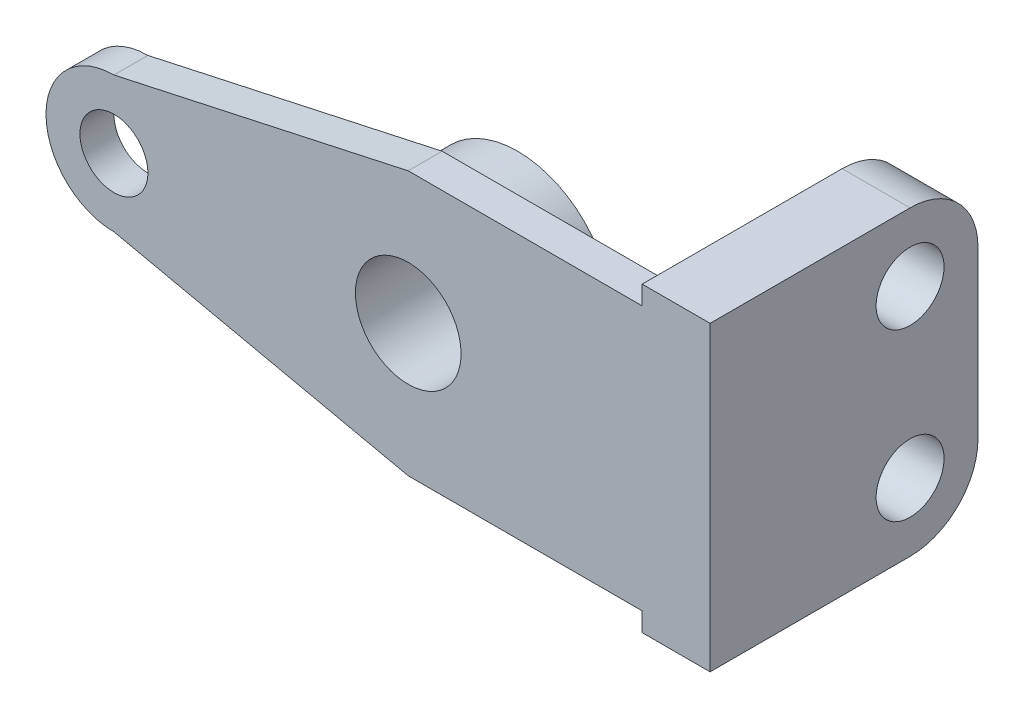
ISO-10303-21;
HEADER;
FILE_DESCRIPTION(('STEP AP214'),'2;1');
FILE_NAME('part.step','',(''),(''),'','','');
FILE_SCHEMA(('AUTOMOTIVE_DESIGN { 1 0 10303 214 1 1 1 1 }'));
ENDSEC;
DATA;
#1=APPLICATION_CONTEXT('core data for automotive mechanical design processes');
#2=APPLICATION_PROTOCOL_DEFINITION('international standard','automotive_design',2000,#1);
#3=PRODUCT_CONTEXT('',#1,'mechanical');
#4=PRODUCT('Part','Part','',(#3));
#5=PRODUCT_RELATED_PRODUCT_CATEGORY('part','',(#4));
#6=PRODUCT_DEFINITION_FORMATION('','',#4);
#7=PRODUCT_DEFINITION_CONTEXT('part definition',#1,'design');
#8=PRODUCT_DEFINITION('design','',#6,#7);
#9=PRODUCT_DEFINITION_SHAPE('','',#8);
#10=(LENGTH_UNIT() NAMED_UNIT(*) SI_UNIT(.MILLI.,.METRE.));
#11=(NAMED_UNIT(*) PLANE_ANGLE_UNIT() SI_UNIT($,.RADIAN.));
#12=(NAMED_UNIT(*) SI_UNIT($,.STERADIAN.) SOLID_ANGLE_UNIT());
#13=UNCERTAINTY_MEASURE_WITH_UNIT(LENGTH_MEASURE(1.E-05),#10,'distance_accuracy_value','');
#14=(GEOMETRIC_REPRESENTATION_CONTEXT(3) GLOBAL_UNCERTAINTY_ASSIGNED_CONTEXT((#13)) GLOBAL_UNIT_ASSIGNED_CONTEXT((#10,
#11,#12)) REPRESENTATION_CONTEXT('',''));
#15=CARTESIAN_POINT('',(0.,0.,0.));
#16=DIRECTION('',(0.,0.,1.));
#17=DIRECTION('',(1.,0.,0.));
#18=AXIS2_PLACEMENT_3D('',#15,#16,#17);
#19=CARTESIAN_POINT('',(-14.5645692766358,66.8256707986819,9.));
#20=DIRECTION('',(-0.212949665458365,0.977063170926614,0.));
#21=DIRECTION('',(-0.977063170926615,-0.212949665458365,0.));
#22=AXIS2_PLACEMENT_3D('',#19,#20,#21);
#23=PLANE('',#22);
#24=DIRECTION('',(0.977063170926614,0.212949665458365,0.));
#25=VECTOR('',#24,1.);
#26=CARTESIAN_POINT('',(-14.5645692766358,66.8256707986819,0.));
#27=LINE('',#26,#25);
#28=CARTESIAN_POINT('',(-78.,53.,0.));
#29=VERTEX_POINT('',#28);
#30=CARTESIAN_POINT('',(0.,70.,0.));
#31=VERTEX_POINT('',#30);
#32=EDGE_CURVE('E206',#29,#31,#27,.T.);
#33=ORIENTED_EDGE('',*,*,#32,.F.);
#34=DIRECTION('',(0.,0.,-1.));
#35=VECTOR('',#34,1.);
#36=CARTESIAN_POINT('',(-78.,53.,9.));
#37=LINE('',#36,#35);
#38=CARTESIAN_POINT('',(-78.,53.,9.));
#39=VERTEX_POINT('',#38);
#40=EDGE_CURVE('E245',#39,#29,#37,.T.);
#41=ORIENTED_EDGE('',*,*,#40,.F.);
#42=DIRECTION('',(0.977063170926614,0.212949665458365,0.));
#43=VECTOR('',#42,1.);
#44=CARTESIAN_POINT('',(-14.5645692766358,66.8256707986819,9.));
#45=LINE('',#44,#43);
#46=CARTESIAN_POINT('',(0.,70.,9.));
#47=VERTEX_POINT('',#46);
#48=EDGE_CURVE('E207',#39,#47,#45,.T.);
#49=ORIENTED_EDGE('',*,*,#48,.T.);
#50=DIRECTION('',(0.,0.,-1.));
#51=VECTOR('',#50,1.);
#52=CARTESIAN_POINT('',(0.,70.,9.));
#53=LINE('',#52,#51);
#54=EDGE_CURVE('E222',#47,#31,#53,.T.);
#55=ORIENTED_EDGE('',*,*,#54,.T.);
#56=EDGE_LOOP('',(#33,#41,#49,#55));
#57=FACE_BOUND('',#56,.T.);
#58=ADVANCED_FACE('F41',(#57),#23,.T.);
#59=CARTESIAN_POINT('',(-78.,35.,9.));
#60=DIRECTION('',(0.,0.,-1.));
#61=DIRECTION('',(-1.,0.,0.));
#62=AXIS2_PLACEMENT_3D('',#59,#60,#61);
#63=CYLINDRICAL_SURFACE('',#62,18.);
#64=CARTESIAN_POINT('',(-78.,35.,0.));
#65=DIRECTION('',(0.,0.,1.));
#66=DIRECTION('',(1.,0.,0.));
#67=AXIS2_PLACEMENT_3D('',#64,#65,#66);
#68=CIRCLE('',#67,18.);
#69=CARTESIAN_POINT('',(-78.,17.,0.));
#70=VERTEX_POINT('',#69);
#71=EDGE_CURVE('E221',#29,#70,#68,.T.);
#72=ORIENTED_EDGE('',*,*,#71,.T.);
#73=DIRECTION('',(0.,0.,-1.));
#74=VECTOR('',#73,1.);
#75=CARTESIAN_POINT('',(-78.,17.,9.));
#76=LINE('',#75,#74);
#77=CARTESIAN_POINT('',(-78.,17.,9.));
#78=VERTEX_POINT('',#77);
#79=EDGE_CURVE('E239',#78,#70,#76,.T.);
#80=ORIENTED_EDGE('',*,*,#79,.F.);
#81=CARTESIAN_POINT('',(-78.,35.,9.));
#82=DIRECTION('',(0.,0.,1.));
#83=DIRECTION('',(1.,0.,0.));
#84=AXIS2_PLACEMENT_3D('',#81,#82,#83);
#85=CIRCLE('',#84,18.);
#86=EDGE_CURVE('E215',#39,#78,#85,.T.);
#87=ORIENTED_EDGE('',*,*,#86,.F.);
#88=ORIENTED_EDGE('',*,*,#40,.T.);
#89=EDGE_LOOP('',(#72,#80,#87,#88));
#90=FACE_BOUND('',#89,.T.);
#91=ADVANCED_FACE('F289',(#90),#63,.T.);
#92=CARTESIAN_POINT('',(0.,0.,9.));
#93=DIRECTION('',(0.212949665458365,0.977063170926614,0.));
#94=DIRECTION('',(-0.977063170926615,0.212949665458365,0.));
#95=AXIS2_PLACEMENT_3D('',#92,#93,#94);
#96=PLANE('',#95);
#97=DIRECTION('',(0.977063170926614,-0.212949665458365,0.));
#98=VECTOR('',#97,1.);
#99=CARTESIAN_POINT('',(0.,0.,0.));
#100=LINE('',#99,#98);
#101=CARTESIAN_POINT('',(0.,0.,0.));
#102=VERTEX_POINT('',#101);
#103=EDGE_CURVE('E227',#70,#102,#100,.T.);
#104=ORIENTED_EDGE('',*,*,#103,.T.);
#105=DIRECTION('',(0.,0.,-1.));
#106=VECTOR('',#105,1.);
#107=CARTESIAN_POINT('',(0.,0.,9.));
#108=LINE('',#107,#106);
#109=CARTESIAN_POINT('',(0.,0.,9.));
#110=VERTEX_POINT('',#109);
#111=EDGE_CURVE('E237',#110,#102,#108,.T.);
#112=ORIENTED_EDGE('',*,*,#111,.F.);
#113=DIRECTION('',(0.977063170926614,-0.212949665458365,0.));
#114=VECTOR('',#113,1.);
#115=CARTESIAN_POINT('',(0.,0.,9.));
#116=LINE('',#115,#114);
#117=EDGE_CURVE('E214',#78,#110,#116,.T.);
#118=ORIENTED_EDGE('',*,*,#117,.F.);
#119=ORIENTED_EDGE('',*,*,#79,.T.);
#120=EDGE_LOOP('',(#104,#112,#118,#119));
#121=FACE_BOUND('',#120,.T.);
#122=ADVANCED_FACE('F292',(#121),#96,.F.);
#123=CARTESIAN_POINT('',(0.,0.,9.));
#124=DIRECTION('',(0.,1.,0.));
#125=DIRECTION('',(0.,0.,1.));
#126=AXIS2_PLACEMENT_3D('',#123,#124,#125);
#127=PLANE('',#126);
#128=DIRECTION('',(1.,0.,0.));
#129=VECTOR('',#128,1.);
#130=CARTESIAN_POINT('',(0.,0.,0.));
#131=LINE('',#130,#129);
#132=CARTESIAN_POINT('',(62.,0.,0.));
#133=VERTEX_POINT('',#132);
#134=EDGE_CURVE('E228',#102,#133,#131,.T.);
#135=ORIENTED_EDGE('',*,*,#134,.T.);
#136=DIRECTION('',(0.,0.,1.));
#137=VECTOR('',#136,1.);
#138=CARTESIAN_POINT('',(62.,0.,9.));
#139=LINE('',#138,#137);
#140=CARTESIAN_POINT('',(62.,0.,9.));
#141=VERTEX_POINT('',#140);
#142=EDGE_CURVE('E63',#133,#141,#139,.T.);
#143=ORIENTED_EDGE('',*,*,#142,.T.);
#144=DIRECTION('',(1.,0.,0.));
#145=VECTOR('',#144,1.);
#146=CARTESIAN_POINT('',(0.,0.,9.));
#147=LINE('',#146,#145);
#148=EDGE_CURVE('E136',#110,#141,#147,.T.);
#149=ORIENTED_EDGE('',*,*,#148,.F.);
#150=ORIENTED_EDGE('',*,*,#111,.T.);
#151=EDGE_LOOP('',(#135,#143,#149,#150));
#152=FACE_BOUND('',#151,.T.);
#153=ADVANCED_FACE('F305',(#152),#127,.F.);
#154=CARTESIAN_POINT('',(80.,0.,9.));
#155=DIRECTION('',(1.,0.,0.));
#156=DIRECTION('',(0.,0.,-1.));
#157=AXIS2_PLACEMENT_3D('',#154,#155,#156);
#158=PLANE('',#157);
#159=CARTESIAN_POINT('',(80.,57.,-44.));
#160=DIRECTION('',(1.,0.,0.));
#161=DIRECTION('',(0.,0.,-1.));
#162=AXIS2_PLACEMENT_3D('',#159,#160,#161);
#163=CIRCLE('',#162,9.);
#164=CARTESIAN_POINT('',(80.,57.,-53.));
#165=VERTEX_POINT('',#164);
#166=EDGE_CURVE('E452',#165,#165,#163,.T.);
#167=ORIENTED_EDGE('',*,*,#166,.F.);
#168=EDGE_LOOP('',(#167));
#169=FACE_BOUND('',#168,.T.);
#170=CARTESIAN_POINT('',(80.,13.,-44.));
#171=DIRECTION('',(1.,0.,0.));
#172=DIRECTION('',(0.,0.,-1.));
#173=AXIS2_PLACEMENT_3D('',#170,#171,#172);
#174=CIRCLE('',#173,9.);
#175=CARTESIAN_POINT('',(80.,13.,-53.));
#176=VERTEX_POINT('',#175);
#177=EDGE_CURVE('E457',#176,#176,#174,.T.);
#178=ORIENTED_EDGE('',*,*,#177,.F.);
#179=EDGE_LOOP('',(#178));
#180=FACE_BOUND('',#179,.T.);
#181=DIRECTION('',(0.,0.,-1.));
#182=VECTOR('',#181,1.);
#183=CARTESIAN_POINT('',(80.,-5.,9.));
#184=LINE('',#183,#182);
#185=CARTESIAN_POINT('',(80.,-5.,9.));
#186=VERTEX_POINT('',#185);
#187=CARTESIAN_POINT('',(80.,-5.,-44.));
#188=VERTEX_POINT('',#187);
#189=EDGE_CURVE('E146',#186,#188,#184,.T.);
#190=ORIENTED_EDGE('',*,*,#189,.T.);
#191=CARTESIAN_POINT('',(80.,13.,-44.));
#192=DIRECTION('',(1.,0.,0.));
#193=DIRECTION('',(0.,0.,1.));
#194=AXIS2_PLACEMENT_3D('',#191,#192,#193);
#195=CIRCLE('',#194,18.);
#196=CARTESIAN_POINT('',(80.,13.,-62.));
#197=VERTEX_POINT('',#196);
#198=EDGE_CURVE('E168',#188,#197,#195,.T.);
#199=ORIENTED_EDGE('',*,*,#198,.T.);
#200=DIRECTION('',(0.,1.,0.));
#201=VECTOR('',#200,1.);
#202=CARTESIAN_POINT('',(80.,57.,-62.));
#203=LINE('',#202,#201);
#204=CARTESIAN_POINT('',(80.,57.,-62.));
#205=VERTEX_POINT('',#204);
#206=EDGE_CURVE('E173',#197,#205,#203,.T.);
#207=ORIENTED_EDGE('',*,*,#206,.T.);
#208=CARTESIAN_POINT('',(80.,57.,-44.));
#209=DIRECTION('',(1.,0.,0.));
#210=DIRECTION('',(0.,0.,1.));
#211=AXIS2_PLACEMENT_3D('',#208,#209,#210);
#212=CIRCLE('',#211,18.);
#213=CARTESIAN_POINT('',(80.,75.,-44.));
#214=VERTEX_POINT('',#213);
#215=EDGE_CURVE('E143',#205,#214,#212,.T.);
#216=ORIENTED_EDGE('',*,*,#215,.T.);
#217=DIRECTION('',(0.,0.,-1.));
#218=VECTOR('',#217,1.);
#219=CARTESIAN_POINT('',(80.,75.,9.));
#220=LINE('',#219,#218);
#221=CARTESIAN_POINT('',(80.,75.,9.));
#222=VERTEX_POINT('',#221);
#223=EDGE_CURVE('E235',#222,#214,#220,.T.);
#224=ORIENTED_EDGE('',*,*,#223,.F.);
#225=DIRECTION('',(0.,-1.,0.));
#226=VECTOR('',#225,1.);
#227=CARTESIAN_POINT('',(80.,0.,9.));
#228=LINE('',#227,#226);
#229=EDGE_CURVE('E217',#222,#186,#228,.T.);
#230=ORIENTED_EDGE('',*,*,#229,.T.);
#231=EDGE_LOOP('',(#190,#199,#207,#216,#224,#230));
#232=FACE_BOUND('',#231,.T.);
#233=ADVANCED_FACE('F274',(#169,#180,#232),#158,.T.);
#234=CARTESIAN_POINT('',(0.,70.,9.));
#235=DIRECTION('',(0.,1.,0.));
#236=DIRECTION('',(0.,0.,1.));
#237=AXIS2_PLACEMENT_3D('',#234,#235,#236);
#238=PLANE('',#237);
#239=DIRECTION('',(0.,0.,1.));
#240=VECTOR('',#239,1.);
#241=CARTESIAN_POINT('',(62.,70.,9.));
#242=LINE('',#241,#240);
#243=CARTESIAN_POINT('',(62.,70.,0.));
#244=VERTEX_POINT('',#243);
#245=CARTESIAN_POINT('',(62.,70.,9.));
#246=VERTEX_POINT('',#245);
#247=EDGE_CURVE('E185',#244,#246,#242,.T.);
#248=ORIENTED_EDGE('',*,*,#247,.F.);
#249=DIRECTION('',(1.,0.,0.));
#250=VECTOR('',#249,1.);
#251=CARTESIAN_POINT('',(0.,70.,0.));
#252=LINE('',#251,#250);
#253=EDGE_CURVE('E213',#31,#244,#252,.T.);
#254=ORIENTED_EDGE('',*,*,#253,.F.);
#255=ORIENTED_EDGE('',*,*,#54,.F.);
#256=DIRECTION('',(1.,0.,0.));
#257=VECTOR('',#256,1.);
#258=CARTESIAN_POINT('',(0.,70.,9.));
#259=LINE('',#258,#257);
#260=EDGE_CURVE('E54',#47,#246,#259,.T.);
#261=ORIENTED_EDGE('',*,*,#260,.T.);
#262=EDGE_LOOP('',(#248,#254,#255,#261));
#263=FACE_BOUND('',#262,.T.);
#264=ADVANCED_FACE('F294',(#263),#238,.T.);
#265=CARTESIAN_POINT('',(0.,0.,9.));
#266=DIRECTION('',(0.,0.,1.));
#267=DIRECTION('',(1.,0.,0.));
#268=AXIS2_PLACEMENT_3D('',#265,#266,#267);
#269=PLANE('',#268);
#270=ORIENTED_EDGE('',*,*,#229,.F.);
#271=DIRECTION('',(1.,0.,0.));
#272=VECTOR('',#271,1.);
#273=CARTESIAN_POINT('',(62.,75.,9.));
#274=LINE('',#273,#272);
#275=CARTESIAN_POINT('',(62.,75.,9.));
#276=VERTEX_POINT('',#275);
#277=EDGE_CURVE('E178',#276,#222,#274,.T.);
#278=ORIENTED_EDGE('',*,*,#277,.F.);
#279=DIRECTION('',(0.,-1.,0.));
#280=VECTOR('',#279,1.);
#281=CARTESIAN_POINT('',(62.,-5.,9.));
#282=LINE('',#281,#280);
#283=EDGE_CURVE('E137',#276,#246,#282,.T.);
#284=ORIENTED_EDGE('',*,*,#283,.T.);
#285=ORIENTED_EDGE('',*,*,#260,.F.);
#286=ORIENTED_EDGE('',*,*,#48,.F.);
#287=ORIENTED_EDGE('',*,*,#86,.T.);
#288=ORIENTED_EDGE('',*,*,#117,.T.);
#289=ORIENTED_EDGE('',*,*,#148,.T.);
#290=CARTESIAN_POINT('',(62.,-5.,9.));
#291=VERTEX_POINT('',#290);
#292=EDGE_CURVE('E128',#141,#291,#282,.T.);
#293=ORIENTED_EDGE('',*,*,#292,.T.);
#294=DIRECTION('',(1.,0.,0.));
#295=VECTOR('',#294,1.);
#296=CARTESIAN_POINT('',(62.,-5.,9.));
#297=LINE('',#296,#295);
#298=EDGE_CURVE('E131',#291,#186,#297,.T.);
#299=ORIENTED_EDGE('',*,*,#298,.T.);
#300=EDGE_LOOP('',(#270,#278,#284,#285,#286,#287,#288,#289,#293,#299));
#301=FACE_BOUND('',#300,.T.);
#302=CARTESIAN_POINT('',(0.,35.,9.));
#303=DIRECTION('',(0.,0.,-1.));
#304=DIRECTION('',(-1.,0.,0.));
#305=AXIS2_PLACEMENT_3D('',#302,#303,#304);
#306=CIRCLE('',#305,14.);
#307=CARTESIAN_POINT('',(-14.,35.,9.));
#308=VERTEX_POINT('',#307);
#309=EDGE_CURVE('E193',#308,#308,#306,.T.);
#310=ORIENTED_EDGE('',*,*,#309,.T.);
#311=EDGE_LOOP('',(#310));
#312=FACE_BOUND('',#311,.T.);
#313=CARTESIAN_POINT('',(-78.,35.,9.));
#314=DIRECTION('',(0.,0.,-1.));
#315=DIRECTION('',(-1.,0.,0.));
#316=AXIS2_PLACEMENT_3D('',#313,#314,#315);
#317=CIRCLE('',#316,9.);
#318=CARTESIAN_POINT('',(-87.,35.,9.));
#319=VERTEX_POINT('',#318);
#320=EDGE_CURVE('E201',#319,#319,#317,.T.);
#321=ORIENTED_EDGE('',*,*,#320,.T.);
#322=EDGE_LOOP('',(#321));
#323=FACE_BOUND('',#322,.T.);
#324=ADVANCED_FACE('F133',(#301,#312,#323),#269,.T.);
#325=CARTESIAN_POINT('',(0.,0.,0.));
#326=DIRECTION('',(0.,0.,1.));
#327=DIRECTION('',(1.,0.,0.));
#328=AXIS2_PLACEMENT_3D('',#325,#326,#327);
#329=PLANE('',#328);
#330=CARTESIAN_POINT('',(0.,35.,0.));
#331=DIRECTION('',(0.,0.,1.));
#332=DIRECTION('',(1.,0.,0.));
#333=AXIS2_PLACEMENT_3D('',#330,#331,#332);
#334=CIRCLE('',#333,25.);
#335=CARTESIAN_POINT('',(25.,35.,0.));
#336=VERTEX_POINT('',#335);
#337=EDGE_CURVE('E48',#336,#336,#334,.F.);
#338=ORIENTED_EDGE('',*,*,#337,.F.);
#339=EDGE_LOOP('',(#338));
#340=FACE_BOUND('',#339,.T.);
#341=CARTESIAN_POINT('',(-78.,35.,0.));
#342=DIRECTION('',(0.,0.,-1.));
#343=DIRECTION('',(-1.,0.,0.));
#344=AXIS2_PLACEMENT_3D('',#341,#342,#343);
#345=CIRCLE('',#344,9.);
#346=CARTESIAN_POINT('',(-87.,35.,0.));
#347=VERTEX_POINT('',#346);
#348=EDGE_CURVE('E205',#347,#347,#345,.T.);
#349=ORIENTED_EDGE('',*,*,#348,.F.);
#350=EDGE_LOOP('',(#349));
#351=FACE_BOUND('',#350,.T.);
#352=ORIENTED_EDGE('',*,*,#253,.T.);
#353=DIRECTION('',(0.,-1.,0.));
#354=VECTOR('',#353,1.);
#355=CARTESIAN_POINT('',(62.,0.,0.));
#356=LINE('',#355,#354);
#357=EDGE_CURVE('E11',#244,#133,#356,.T.);
#358=ORIENTED_EDGE('',*,*,#357,.T.);
#359=ORIENTED_EDGE('',*,*,#134,.F.);
#360=ORIENTED_EDGE('',*,*,#103,.F.);
#361=ORIENTED_EDGE('',*,*,#71,.F.);
#362=ORIENTED_EDGE('',*,*,#32,.T.);
#363=EDGE_LOOP('',(#352,#358,#359,#360,#361,#362));
#364=FACE_BOUND('',#363,.T.);
#365=ADVANCED_FACE('F250',(#340,#351,#364),#329,.F.);
#366=CARTESIAN_POINT('',(-78.,35.,9.));
#367=DIRECTION('',(0.,0.,-1.));
#368=DIRECTION('',(-1.,0.,0.));
#369=AXIS2_PLACEMENT_3D('',#366,#367,#368);
#370=CYLINDRICAL_SURFACE('',#369,9.);
#371=ORIENTED_EDGE('',*,*,#320,.F.);
#372=EDGE_LOOP('',(#371));
#373=FACE_BOUND('',#372,.T.);
#374=ORIENTED_EDGE('',*,*,#348,.T.);
#375=EDGE_LOOP('',(#374));
#376=FACE_BOUND('',#375,.T.);
#377=ADVANCED_FACE('F253',(#373,#376),#370,.F.);
#378=CARTESIAN_POINT('',(0.,35.,-20.));
#379=DIRECTION('',(0.,0.,1.));
#380=DIRECTION('',(1.,0.,0.));
#381=AXIS2_PLACEMENT_3D('',#378,#379,#380);
#382=CYLINDRICAL_SURFACE('',#381,25.);
#383=CARTESIAN_POINT('',(0.,35.,-20.));
#384=DIRECTION('',(0.,0.,-1.));
#385=DIRECTION('',(-1.,0.,0.));
#386=AXIS2_PLACEMENT_3D('',#383,#384,#385);
#387=CIRCLE('',#386,25.);
#388=CARTESIAN_POINT('',(-25.,35.,-20.));
#389=VERTEX_POINT('',#388);
#390=EDGE_CURVE('E197',#389,#389,#387,.T.);
#391=ORIENTED_EDGE('',*,*,#390,.F.);
#392=EDGE_LOOP('',(#391));
#393=FACE_BOUND('',#392,.T.);
#394=ORIENTED_EDGE('',*,*,#337,.T.);
#395=EDGE_LOOP('',(#394));
#396=FACE_BOUND('',#395,.T.);
#397=ADVANCED_FACE('F249',(#393,#396),#382,.T.);
#398=CARTESIAN_POINT('',(0.,35.,-20.));
#399=DIRECTION('',(0.,0.,-1.));
#400=DIRECTION('',(-1.,0.,0.));
#401=AXIS2_PLACEMENT_3D('',#398,#399,#400);
#402=PLANE('',#401);
#403=CARTESIAN_POINT('',(0.,35.,-20.));
#404=DIRECTION('',(0.,0.,-1.));
#405=DIRECTION('',(-1.,0.,0.));
#406=AXIS2_PLACEMENT_3D('',#403,#404,#405);
#407=CIRCLE('',#406,14.);
#408=CARTESIAN_POINT('',(-14.,35.,-20.));
#409=VERTEX_POINT('',#408);
#410=EDGE_CURVE('E195',#409,#409,#407,.T.);
#411=ORIENTED_EDGE('',*,*,#410,.F.);
#412=EDGE_LOOP('',(#411));
#413=FACE_BOUND('',#412,.T.);
#414=ORIENTED_EDGE('',*,*,#390,.T.);
#415=EDGE_LOOP('',(#414));
#416=FACE_BOUND('',#415,.T.);
#417=ADVANCED_FACE('F333',(#413,#416),#402,.T.);
#418=CARTESIAN_POINT('',(0.,35.,9.));
#419=DIRECTION('',(0.,0.,-1.));
#420=DIRECTION('',(-1.,0.,0.));
#421=AXIS2_PLACEMENT_3D('',#418,#419,#420);
#422=CYLINDRICAL_SURFACE('',#421,14.);
#423=ORIENTED_EDGE('',*,*,#309,.F.);
#424=EDGE_LOOP('',(#423));
#425=FACE_BOUND('',#424,.T.);
#426=ORIENTED_EDGE('',*,*,#410,.T.);
#427=EDGE_LOOP('',(#426));
#428=FACE_BOUND('',#427,.T.);
#429=ADVANCED_FACE('F343',(#425,#428),#422,.F.);
#430=CARTESIAN_POINT('',(62.,57.,-44.));
#431=DIRECTION('',(-1.,0.,0.));
#432=DIRECTION('',(0.,0.,1.));
#433=AXIS2_PLACEMENT_3D('',#430,#431,#432);
#434=PLANE('',#433);
#435=CARTESIAN_POINT('',(62.,57.,-44.));
#436=DIRECTION('',(1.,0.,0.));
#437=DIRECTION('',(0.,0.,-1.));
#438=AXIS2_PLACEMENT_3D('',#435,#436,#437);
#439=CIRCLE('',#438,9.);
#440=CARTESIAN_POINT('',(62.,57.,-53.));
#441=VERTEX_POINT('',#440);
#442=EDGE_CURVE('E174',#441,#441,#439,.T.);
#443=ORIENTED_EDGE('',*,*,#442,.T.);
#444=EDGE_LOOP('',(#443));
#445=FACE_BOUND('',#444,.T.);
#446=CARTESIAN_POINT('',(62.,13.,-44.));
#447=DIRECTION('',(1.,0.,0.));
#448=DIRECTION('',(0.,0.,-1.));
#449=AXIS2_PLACEMENT_3D('',#446,#447,#448);
#450=CIRCLE('',#449,9.);
#451=CARTESIAN_POINT('',(62.,13.,-53.));
#452=VERTEX_POINT('',#451);
#453=EDGE_CURVE('E453',#452,#452,#450,.T.);
#454=ORIENTED_EDGE('',*,*,#453,.T.);
#455=EDGE_LOOP('',(#454));
#456=FACE_BOUND('',#455,.T.);
#457=ORIENTED_EDGE('',*,*,#142,.F.);
#458=ORIENTED_EDGE('',*,*,#357,.F.);
#459=ORIENTED_EDGE('',*,*,#247,.T.);
#460=ORIENTED_EDGE('',*,*,#283,.F.);
#461=DIRECTION('',(0.,0.,1.));
#462=VECTOR('',#461,1.);
#463=CARTESIAN_POINT('',(62.,75.,9.));
#464=LINE('',#463,#462);
#465=CARTESIAN_POINT('',(62.,75.,-44.));
#466=VERTEX_POINT('',#465);
#467=EDGE_CURVE('E147',#466,#276,#464,.T.);
#468=ORIENTED_EDGE('',*,*,#467,.F.);
#469=CARTESIAN_POINT('',(62.,57.,-44.));
#470=DIRECTION('',(1.,0.,0.));
#471=DIRECTION('',(0.,0.,1.));
#472=AXIS2_PLACEMENT_3D('',#469,#470,#471);
#473=CIRCLE('',#472,18.);
#474=CARTESIAN_POINT('',(62.,57.,-62.));
#475=VERTEX_POINT('',#474);
#476=EDGE_CURVE('E164',#475,#466,#473,.T.);
#477=ORIENTED_EDGE('',*,*,#476,.F.);
#478=DIRECTION('',(0.,1.,0.));
#479=VECTOR('',#478,1.);
#480=CARTESIAN_POINT('',(62.,57.,-62.));
#481=LINE('',#480,#479);
#482=CARTESIAN_POINT('',(62.,13.,-62.));
#483=VERTEX_POINT('',#482);
#484=EDGE_CURVE('E158',#483,#475,#481,.T.);
#485=ORIENTED_EDGE('',*,*,#484,.F.);
#486=CARTESIAN_POINT('',(62.,13.,-44.));
#487=DIRECTION('',(1.,0.,0.));
#488=DIRECTION('',(0.,0.,1.));
#489=AXIS2_PLACEMENT_3D('',#486,#487,#488);
#490=CIRCLE('',#489,18.);
#491=CARTESIAN_POINT('',(62.,-5.,-44.));
#492=VERTEX_POINT('',#491);
#493=EDGE_CURVE('E156',#492,#483,#490,.T.);
#494=ORIENTED_EDGE('',*,*,#493,.F.);
#495=DIRECTION('',(0.,0.,-1.));
#496=VECTOR('',#495,1.);
#497=CARTESIAN_POINT('',(62.,-5.,-44.));
#498=LINE('',#497,#496);
#499=EDGE_CURVE('E150',#291,#492,#498,.T.);
#500=ORIENTED_EDGE('',*,*,#499,.F.);
#501=ORIENTED_EDGE('',*,*,#292,.F.);
#502=EDGE_LOOP('',(#457,#458,#459,#460,#468,#477,#485,#494,#500,#501));
#503=FACE_BOUND('',#502,.T.);
#504=ADVANCED_FACE('F153',(#445,#456,#503),#434,.T.);
#505=CARTESIAN_POINT('',(62.,75.,9.));
#506=DIRECTION('',(0.,1.,0.));
#507=DIRECTION('',(0.,0.,1.));
#508=AXIS2_PLACEMENT_3D('',#505,#506,#507);
#509=PLANE('',#508);
#510=ORIENTED_EDGE('',*,*,#223,.T.);
#511=DIRECTION('',(1.,0.,0.));
#512=VECTOR('',#511,1.);
#513=CARTESIAN_POINT('',(62.,75.,-44.));
#514=LINE('',#513,#512);
#515=EDGE_CURVE('E181',#466,#214,#514,.T.);
#516=ORIENTED_EDGE('',*,*,#515,.F.);
#517=ORIENTED_EDGE('',*,*,#467,.T.);
#518=ORIENTED_EDGE('',*,*,#277,.T.);
#519=EDGE_LOOP('',(#510,#516,#517,#518));
#520=FACE_BOUND('',#519,.T.);
#521=ADVANCED_FACE('F262',(#520),#509,.T.);
#522=CARTESIAN_POINT('',(62.,57.,-44.));
#523=DIRECTION('',(1.,0.,0.));
#524=DIRECTION('',(0.,0.,-1.));
#525=AXIS2_PLACEMENT_3D('',#522,#523,#524);
#526=CYLINDRICAL_SURFACE('',#525,18.);
#527=ORIENTED_EDGE('',*,*,#215,.F.);
#528=DIRECTION('',(1.,0.,0.));
#529=VECTOR('',#528,1.);
#530=CARTESIAN_POINT('',(62.,57.,-62.));
#531=LINE('',#530,#529);
#532=EDGE_CURVE('E187',#475,#205,#531,.T.);
#533=ORIENTED_EDGE('',*,*,#532,.F.);
#534=ORIENTED_EDGE('',*,*,#476,.T.);
#535=ORIENTED_EDGE('',*,*,#515,.T.);
#536=EDGE_LOOP('',(#527,#533,#534,#535));
#537=FACE_BOUND('',#536,.T.);
#538=ADVANCED_FACE('F277',(#537),#526,.T.);
#539=CARTESIAN_POINT('',(62.,57.,-62.));
#540=DIRECTION('',(0.,0.,-1.));
#541=DIRECTION('',(-1.,0.,0.));
#542=AXIS2_PLACEMENT_3D('',#539,#540,#541);
#543=PLANE('',#542);
#544=ORIENTED_EDGE('',*,*,#206,.F.);
#545=DIRECTION('',(1.,0.,0.));
#546=VECTOR('',#545,1.);
#547=CARTESIAN_POINT('',(62.,13.,-62.));
#548=LINE('',#547,#546);
#549=EDGE_CURVE('E188',#483,#197,#548,.T.);
#550=ORIENTED_EDGE('',*,*,#549,.F.);
#551=ORIENTED_EDGE('',*,*,#484,.T.);
#552=ORIENTED_EDGE('',*,*,#532,.T.);
#553=EDGE_LOOP('',(#544,#550,#551,#552));
#554=FACE_BOUND('',#553,.T.);
#555=ADVANCED_FACE('F267',(#554),#543,.T.);
#556=CARTESIAN_POINT('',(62.,13.,-44.));
#557=DIRECTION('',(1.,0.,0.));
#558=DIRECTION('',(0.,0.,-1.));
#559=AXIS2_PLACEMENT_3D('',#556,#557,#558);
#560=CYLINDRICAL_SURFACE('',#559,18.);
#561=ORIENTED_EDGE('',*,*,#198,.F.);
#562=DIRECTION('',(1.,0.,0.));
#563=VECTOR('',#562,1.);
#564=CARTESIAN_POINT('',(62.,-5.,-44.));
#565=LINE('',#564,#563);
#566=EDGE_CURVE('E149',#492,#188,#565,.T.);
#567=ORIENTED_EDGE('',*,*,#566,.F.);
#568=ORIENTED_EDGE('',*,*,#493,.T.);
#569=ORIENTED_EDGE('',*,*,#549,.T.);
#570=EDGE_LOOP('',(#561,#567,#568,#569));
#571=FACE_BOUND('',#570,.T.);
#572=ADVANCED_FACE('F272',(#571),#560,.T.);
#573=CARTESIAN_POINT('',(62.,-5.,-44.));
#574=DIRECTION('',(0.,-1.,0.));
#575=DIRECTION('',(0.,0.,-1.));
#576=AXIS2_PLACEMENT_3D('',#573,#574,#575);
#577=PLANE('',#576);
#578=ORIENTED_EDGE('',*,*,#189,.F.);
#579=ORIENTED_EDGE('',*,*,#298,.F.);
#580=ORIENTED_EDGE('',*,*,#499,.T.);
#581=ORIENTED_EDGE('',*,*,#566,.T.);
#582=EDGE_LOOP('',(#578,#579,#580,#581));
#583=FACE_BOUND('',#582,.T.);
#584=ADVANCED_FACE('F144',(#583),#577,.T.);
#585=CARTESIAN_POINT('',(62.,13.,-44.));
#586=DIRECTION('',(1.,0.,0.));
#587=DIRECTION('',(0.,0.,-1.));
#588=AXIS2_PLACEMENT_3D('',#585,#586,#587);
#589=CYLINDRICAL_SURFACE('',#588,9.);
#590=ORIENTED_EDGE('',*,*,#453,.F.);
#591=EDGE_LOOP('',(#590));
#592=FACE_BOUND('',#591,.T.);
#593=ORIENTED_EDGE('',*,*,#177,.T.);
#594=EDGE_LOOP('',(#593));
#595=FACE_BOUND('',#594,.T.);
#596=ADVANCED_FACE('F421',(#592,#595),#589,.F.);
#597=CARTESIAN_POINT('',(62.,57.,-44.));
#598=DIRECTION('',(1.,0.,0.));
#599=DIRECTION('',(0.,0.,-1.));
#600=AXIS2_PLACEMENT_3D('',#597,#598,#599);
#601=CYLINDRICAL_SURFACE('',#600,9.);
#602=ORIENTED_EDGE('',*,*,#442,.F.);
#603=EDGE_LOOP('',(#602));
#604=FACE_BOUND('',#603,.T.);
#605=ORIENTED_EDGE('',*,*,#166,.T.);
#606=EDGE_LOOP('',(#605));
#607=FACE_BOUND('',#606,.T.);
#608=ADVANCED_FACE('F435',(#604,#607),#601,.F.);
#609=CLOSED_SHELL('',(#58,#91,#122,#153,#233,#264,#324,#365,#377,#397,#417,#429,#504,#521,#538,
#555,#572,#584,#596,#608));
#610=MANIFOLD_SOLID_BREP('B2',#609);
#611=ADVANCED_BREP_SHAPE_REPRESENTATION('',(#18,#610),#14);
#612=SHAPE_DEFINITION_REPRESENTATION(#9,#611);
ENDSEC;
END-ISO-10303-21;
